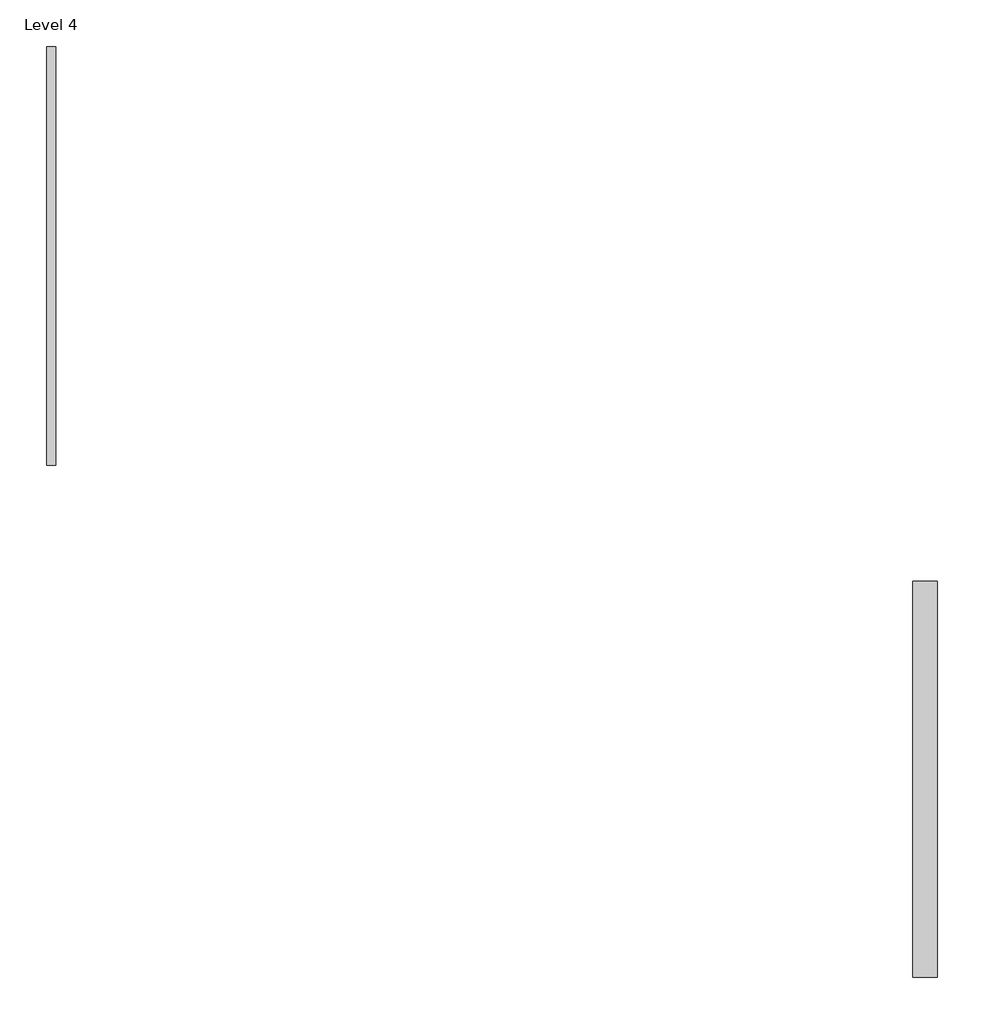
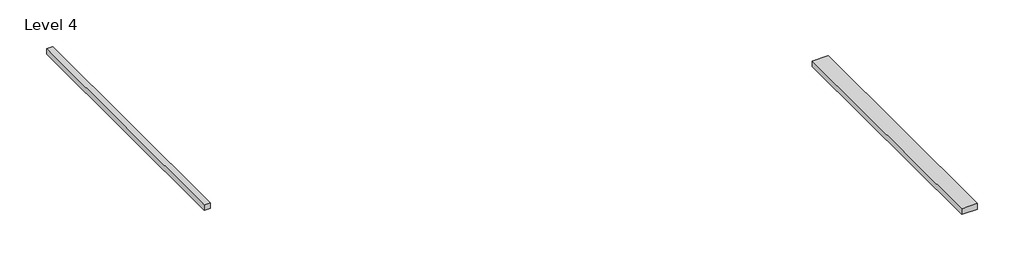
# One storey: 2 proxies.
"""IFC4 building model written with IfcOpenShell, lengths in millimetres."""

from ifc_helpers import new_model, si_unit, origin, place, context, project, spatial, transform, mapped, element, save
from components import generic_models_11_generic_models_11_f4245121, generic_models_5_generic_models_4_07a2a312

model = new_model("IFC4")

# Units and contexts
model_context = context("Model", 3, world=origin())
ifc_project = project(units=[si_unit("LENGTHUNIT", "METRE", prefix="MILLI")], contexts=[model_context])

# Site, building, storey
site = spatial("IfcSite", under=ifc_project)
building = spatial("IfcBuilding", under=site)
storey = spatial("IfcBuildingStorey", under=building, Name="Level 4", Elevation=9144.0)

# Proxies
placement = place(None, origin())
generic_models_11_generic_models_11_shape = generic_models_11_generic_models_11_f4245121(model_context)
element("IfcBuildingElementProxy", 1, Name="Generic Models 11 : Generic Models 11", ObjectType="Generic Models 11 : Generic Models 11", at=placement, inside=storey, context=model_context, shape_type="MappedRepresentation", body=[
    mapped(generic_models_11_generic_models_11_shape, transform((0.0, 0.0, 0.0), x_axis=(1.0, 0.0, 0.0), y_axis=(0.0, 1.0, 0.0), z_axis=(0.0, 0.0, 1.0))),
])
generic_models_5_generic_models_4_shape = generic_models_5_generic_models_4_07a2a312(model_context)
element("IfcBuildingElementProxy", 2, Name="Generic Models 5 : Generic Models 4", ObjectType="Generic Models 5 : Generic Models 4", at=placement, inside=storey, context=model_context, shape_type="MappedRepresentation", body=[
    mapped(generic_models_5_generic_models_4_shape, transform((0.0, -32.6595923, 3067.6539272), x_axis=(1.0, 0.0, 0.0), y_axis=(0.0, 1.0, 0.0), z_axis=(0.0, 0.0, 1.0))),
])

save(model, "model.ifc")

# Revit data of these elements
# Element 1 (IfcBuildingElementProxy, "Generic Models 11 : Generic Models 11")
#   Phase Created = New Construction
# Element 2 (IfcBuildingElementProxy, "Generic Models 5 : Generic Models 4")
#   Phase Created = New Construction
